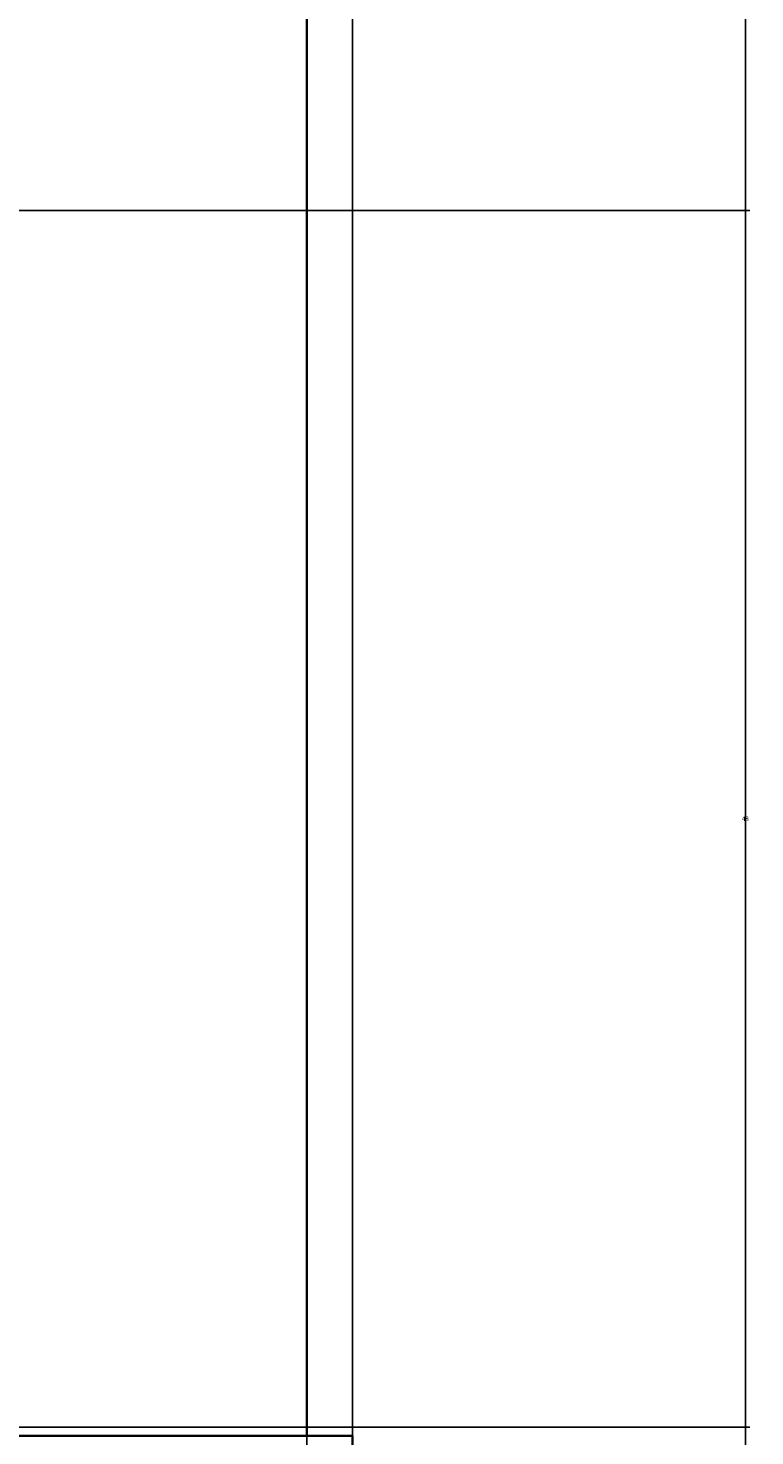
# Model space of a CAD drawing. Units: inches. Extents: x -6 to 289, y -8 to 323.
# Tile 41 of 107: x 260 to 289, y 68 to 124. Entities that reach past the tile are written whole.
import ezdxf

# ---------------------------------------------------------------- set-up
doc = ezdxf.new("R2010")
doc.units = ezdxf.units.IN
doc.header["$MEASUREMENT"] = 0
doc.layers.add('A-ANNO-DIMS', color=2, linetype='Continuous', lineweight=18)
doc.layers.add('A-ELEV', color=7, linetype='Continuous', lineweight=35)
doc.styles.get("Standard").update_dxf_attribs({"font": 'arial.ttf'})
doc.dimstyles.get("Standard").update_dxf_attribs({"dimtxt": 0.18, "dimasz": 0.18, "dimexe": 0.18, "dimexo": 0.0625, "dimgap": 0.09, "dimtad": 0, "dimtih": 1, "dimtoh": 1, "dimdec": 4, "dimzin": 0, "dimdsep": 46, "dimtxsty": 'Standard', "dimcen": 0.09, "dimadec": 0, "dimazin": 0, "dimtfac": 1, "dimtdec": 4, "dimtofl": 0, "dimtmove": 0, "dimatfit": 3, "dimfxl": 1, "dimtolj": 1, "dimtzin": 0, "dimarcsym": 0})

# ---------------------------------------------------------------- blocks, each defined once
blk = doc.blocks.new('*D15')
at = {"layer": 'A-ANNO-DIMS', "color": 0, "lineweight": -2, "transparency": 16777216}
for p, q in [((247.164, 162.411), (247.164, 322.969)), ((247.344, 322.789), (258.944, 322.789)), ((270.984, 322.789), (259.384, 322.789)), ((271.164, 7.351), (271.164, 322.969))]:
    blk.add_line(p, q, dxfattribs=at)
at = {"layer": 'A-ANNO-DIMS', "color": 0, "transparency": 16777216}
for points in [[(247.344, 322.819), (247.344, 322.759), (247.164, 322.789)], [(270.984, 322.819), (270.984, 322.759), (271.164, 322.789)]]:
    blk.add_solid(points, dxfattribs=at)
at = {"layer": 'Defpoints', "color": 0, "transparency": 16777216}
for p in [(271.164, 322.789), (247.164, 162.348), (271.164, 7.289)]:
    blk.add_point(p, dxfattribs=at)
at = {"layer": 'A-ANNO-DIMS', "color": 0, "transparency": 16777216, "insert": (259.164, 322.789), "char_height": 0.18, "attachment_point": 5}
blk.add_mtext('\\A1;24', dxfattribs=at)
blk = doc.blocks.new('*D23')
at = {"layer": 'A-ANNO-DIMS', "color": 0, "lineweight": -2, "transparency": 16777216}
for p, q in [((259.226, 127.289), (288.653, 127.289)), ((288.473, 127.109), (288.473, 67.471)), ((288.473, 7.469), (288.473, 67.107)), ((271.226, 7.289), (288.653, 7.289))]:
    blk.add_line(p, q, dxfattribs=at)
at = {"layer": 'A-ANNO-DIMS', "color": 0, "transparency": 16777216}
for points in [[(288.443, 127.109), (288.503, 127.109), (288.473, 127.289)], [(288.443, 7.469), (288.503, 7.469), (288.473, 7.289)]]:
    blk.add_solid(points, dxfattribs=at)
at = {"layer": 'Defpoints', "color": 0, "transparency": 16777216}
for p in [(259.164, 127.289), (288.473, 127.289), (271.164, 7.289)]:
    blk.add_point(p, dxfattribs=at)
at = {"layer": 'A-ANNO-DIMS', "color": 0, "transparency": 16777216, "insert": (288.473, 67.289), "char_height": 0.18, "attachment_point": 5}
blk.add_mtext('\\A1;120', dxfattribs=at)
blk = doc.blocks.new('*D82')
at = {"layer": 'A-ANNO-DIMS', "color": 0, "lineweight": -2, "transparency": 16777216}
for p, q in [((245.215, 66.286), (245.215, 322.969)), ((245.395, 322.789), (258.699, 322.789)), ((272.793, 322.789), (259.489, 322.789)), ((272.973, 66.286), (272.973, 322.969))]:
    blk.add_line(p, q, dxfattribs=at)
at = {"layer": 'A-ANNO-DIMS', "color": 0, "transparency": 16777216}
for points in [[(245.395, 322.819), (245.395, 322.759), (245.215, 322.789)], [(272.793, 322.819), (272.793, 322.759), (272.973, 322.789)]]:
    blk.add_solid(points, dxfattribs=at)
at = {"layer": 'Defpoints', "color": 0, "transparency": 16777216}
for p in [(272.973, 322.789), (245.215, 66.224), (272.973, 66.224)]:
    blk.add_point(p, dxfattribs=at)
at = {"layer": 'A-ANNO-DIMS', "color": 0, "transparency": 16777216, "insert": (259.094, 322.789), "char_height": 0.18, "attachment_point": 5}
blk.add_mtext('\\A1;27.76', dxfattribs=at)
blk = doc.blocks.new('*D90')
at = {"layer": 'A-ANNO-DIMS', "color": 0, "lineweight": -2, "transparency": 16777216}
for p, q in [((230.354, 68.779), (288.653, 68.779)), ((288.473, 68.599), (288.473, 60.114)), ((288.473, 51.265), (288.473, 59.75)), ((247.303, 51.085), (288.653, 51.085))]:
    blk.add_line(p, q, dxfattribs=at)
at = {"layer": 'A-ANNO-DIMS', "color": 0, "transparency": 16777216}
for points in [[(288.443, 68.599), (288.503, 68.599), (288.473, 68.779)], [(288.443, 51.265), (288.503, 51.265), (288.473, 51.085)]]:
    blk.add_solid(points, dxfattribs=at)
at = {"layer": 'Defpoints', "color": 0, "transparency": 16777216}
for p in [(230.292, 68.779), (288.473, 68.779), (247.241, 51.085)]:
    blk.add_point(p, dxfattribs=at)
at = {"layer": 'A-ANNO-DIMS', "color": 0, "transparency": 16777216, "insert": (288.473, 59.932), "char_height": 0.18, "attachment_point": 5}
blk.add_mtext('\\A1;17.694', dxfattribs=at)
blk = doc.blocks.new('*D91')
at = {"layer": 'A-ANNO-DIMS', "color": 0, "lineweight": -2, "transparency": 16777216}
for p, q in [((230.354, 116.779), (288.653, 116.779)), ((288.473, 116.599), (288.473, 92.961)), ((288.473, 68.959), (288.473, 92.598)), ((230.354, 68.779), (288.653, 68.779))]:
    blk.add_line(p, q, dxfattribs=at)
at = {"layer": 'A-ANNO-DIMS', "color": 0, "transparency": 16777216}
for points in [[(288.443, 116.599), (288.503, 116.599), (288.473, 116.779)], [(288.443, 68.959), (288.503, 68.959), (288.473, 68.779)]]:
    blk.add_solid(points, dxfattribs=at)
at = {"layer": 'Defpoints', "color": 0, "transparency": 16777216}
for p in [(230.292, 116.779), (288.473, 116.779), (230.292, 68.779)]:
    blk.add_point(p, dxfattribs=at)
at = {"layer": 'A-ANNO-DIMS', "color": 0, "transparency": 16777216, "insert": (288.473, 92.779), "char_height": 0.18, "attachment_point": 5}
blk.add_mtext('\\A1;48', dxfattribs=at)

msp = doc.modelspace()

# ---------------------------------------------------------------- linework, layer by layer
at = {"layer": 'A-ELEV'}
msp.add_line((271.1638, 68.4323), (271.1638, 259.2888), dxfattribs=at)
msp.add_lwpolyline([(245.2146, 68.4323), (272.9733, 68.4323), (272.9733, 66.2238), (245.2146, 66.2238)], close=True, dxfattribs=at)

# ---------------------------------------------------------------- dimensions: what is measured, and where the dimension line sits
at = {"layer": 'A-ANNO-DIMS'}
for base, p1, p2, override, picture, middle in [((272.9733, 322.7888), (245.2146, 66.2238), (272.9733, 66.2238), {"dimdec": 2, "dimlfac": 1, "dimrnd": 0, "dimzin": 0, "dimdsep": 46, "dimlunit": 2}, '*D82', (259.0939, 322.7888)), ((271.1638, 322.7888), (247.1638, 162.3484), (271.1638, 7.2888), {"dimdec": 0, "dimlfac": 1, "dimrnd": 0, "dimzin": 0, "dimdsep": 46, "dimlunit": 2}, '*D15', (259.1638, 322.7888))]:
    dim = msp.add_linear_dim(base=base, p1=p1, p2=p2, dimstyle='Standard', override=override, dxfattribs=at)
    dim.commit()
    dim.dimension.update_dxf_attribs({"geometry": picture, "text_midpoint": middle})
for base, p1, p2, override, picture, middle in [((288.4733, 127.2888), (271.1638, 7.2888), (259.1638, 127.2888), {"dimdec": 0, "dimlfac": 1, "dimrnd": 0, "dimzin": 0, "dimdsep": 46, "dimlunit": 2}, '*D23', (288.4733, 67.2888)), ((288.4733, 116.7795), (230.2918, 68.7795), (230.2918, 116.7795), {"dimdec": 0, "dimlfac": 1, "dimrnd": 0, "dimzin": 0, "dimdsep": 46, "dimlunit": 2}, '*D91', (288.4733, 92.7795)), ((288.4733, 68.7795), (247.2408, 51.0851), (230.2918, 68.7795), {"dimdec": 3, "dimlfac": 1, "dimrnd": 0, "dimzin": 0, "dimdsep": 46, "dimlunit": 2}, '*D90', (288.4733, 59.9323))]:
    dim = msp.add_linear_dim(base=base, p1=p1, p2=p2, angle=90, dimstyle='Standard', override=override, dxfattribs=at)
    dim.commit()
    dim.dimension.update_dxf_attribs({"geometry": picture, "text_midpoint": middle})

doc.saveas('drawing.dxf')
